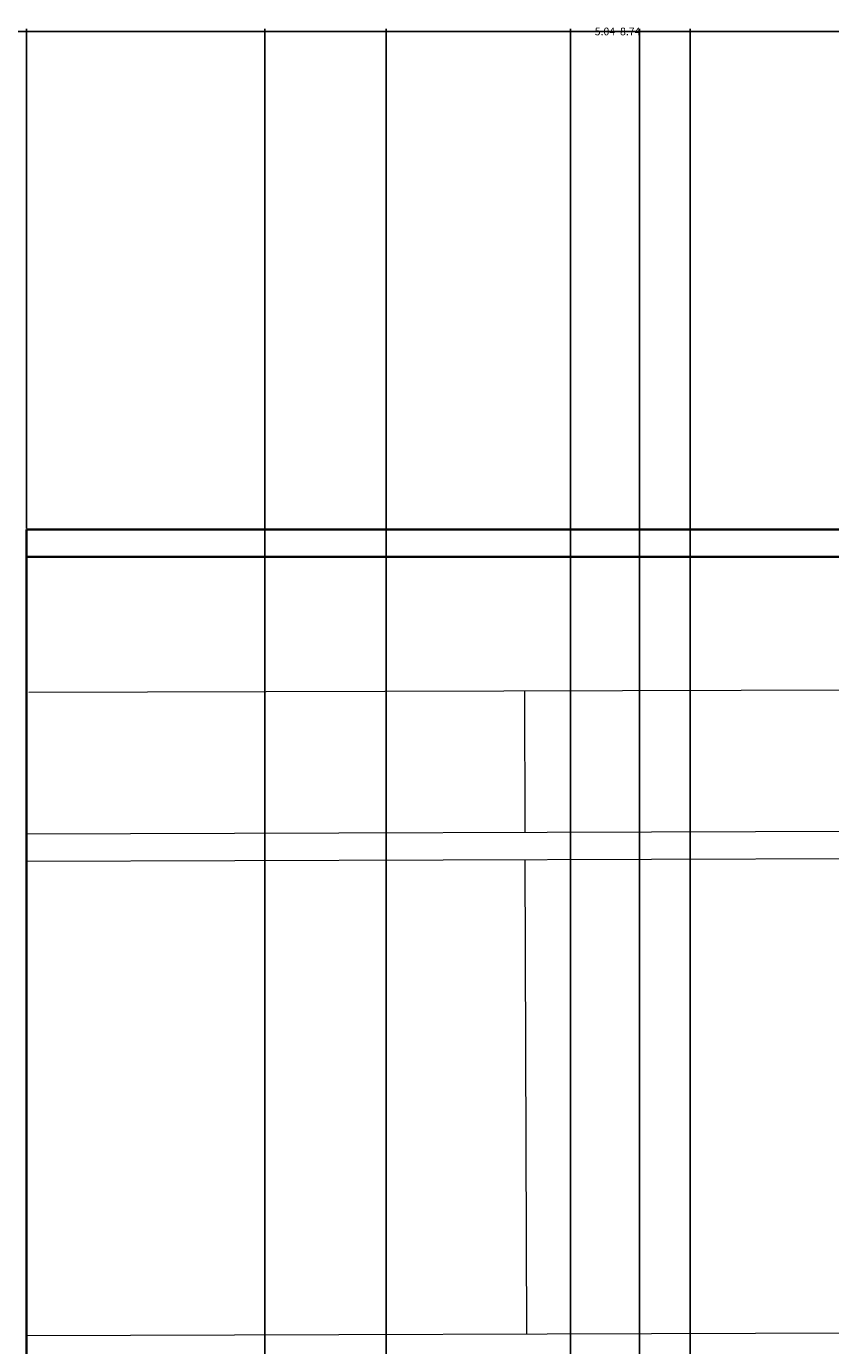
# Model space of a CAD drawing. Units: inches. Extents: x -26 to 776, y -22 to 650.
# Tile 36 of 62: x 192 to 250, y 554 to 650. Entities that reach past the tile are written whole.
import ezdxf

# ---------------------------------------------------------------- set-up
doc = ezdxf.new("R2010")
doc.units = ezdxf.units.IN
doc.header["$MEASUREMENT"] = 0
for name, color, linetype, lineweight in [('A-ANNO-DIMS', 2, 'Continuous', 18), ('A-ROOF', 7, 'Continuous', 35), ('A-WALL', 7, 'Continuous', 35), ('A-WALL-TRIM', 7, 'Continuous', 18)]:
    doc.layers.add(name, color=color, linetype=linetype, lineweight=lineweight)
doc.styles.get("Standard").update_dxf_attribs({"font": 'arial.ttf'})
doc.dimstyles.get("Standard").update_dxf_attribs({"dimtxt": 0.5625, "dimasz": 0.18, "dimexe": 0.18, "dimexo": 0.0625, "dimgap": 0.09, "dimtad": 0, "dimtih": 1, "dimtoh": 1, "dimdec": 4, "dimzin": 0, "dimdsep": 46, "dimlunit": 4, "dimtxsty": 'Standard', "dimcen": 0.09, "dimadec": 0, "dimazin": 0, "dimtfac": 1, "dimtdec": 4, "dimtofl": 0, "dimtmove": 0, "dimatfit": 3, "dimfxl": 1, "dimtolj": 1, "dimtzin": 0, "dimarcsym": 0})

# ---------------------------------------------------------------- blocks, each defined once
blk = doc.blocks.new('*D15')
at = {"layer": 'A-ANNO-DIMS', "color": 0, "lineweight": -2, "transparency": 16777216}
for p, q in [((11.107, 491.489), (11.107, 649.856)), ((11.287, 649.676), (120.222, 649.676)), ((231.245, 649.676), (122.31, 649.676)), ((231.425, 491.489), (231.425, 649.856))]:
    blk.add_line(p, q, dxfattribs=at)
at = {"layer": 'A-ANNO-DIMS', "color": 0, "transparency": 16777216}
for points in [[(11.287, 649.706), (11.287, 649.646), (11.107, 649.676)], [(231.245, 649.706), (231.245, 649.646), (231.425, 649.676)]]:
    blk.add_solid(points, dxfattribs=at)
at = {"layer": 'Defpoints', "color": 0, "transparency": 16777216}
for p in [(231.425, 649.676), (11.107, 491.427), (231.425, 491.427)]:
    blk.add_point(p, dxfattribs=at)
at = {"layer": 'A-ANNO-DIMS', "color": 0, "transparency": 16777216, "insert": (121.266, 649.676), "char_height": 0.5625, "attachment_point": 5}
blk.add_mtext('\\A1;220.3', dxfattribs=at)
blk = doc.blocks.new('*D16')
at = {"layer": 'A-ANNO-DIMS', "color": 0, "lineweight": -2, "transparency": 16777216}
for p, q in [((231.425, 504.483), (231.425, 649.856)), ((231.605, 649.676), (259.297, 649.676)), ((289.062, 649.676), (261.37, 649.676)), ((289.242, 504.483), (289.242, 649.856))]:
    blk.add_line(p, q, dxfattribs=at)
at = {"layer": 'A-ANNO-DIMS', "color": 0, "transparency": 16777216}
for points in [[(231.605, 649.706), (231.605, 649.646), (231.425, 649.676)], [(289.062, 649.706), (289.062, 649.646), (289.242, 649.676)]]:
    blk.add_solid(points, dxfattribs=at)
at = {"layer": 'Defpoints', "color": 0, "transparency": 16777216}
for p in [(289.242, 649.676), (231.425, 504.42), (289.242, 504.42)]:
    blk.add_point(p, dxfattribs=at)
at = {"layer": 'A-ANNO-DIMS', "color": 0, "transparency": 16777216, "insert": (260.334, 649.676), "char_height": 0.5625, "attachment_point": 5}
blk.add_mtext('\\A1;57.82', dxfattribs=at)
blk = doc.blocks.new('*D18')
at = {"layer": 'A-ANNO-DIMS', "color": 0, "lineweight": -2, "transparency": 16777216}
for p, q in [((191.678, 613.334), (191.678, 649.856)), ((191.858, 649.676), (273.361, 649.676)), ((356.887, 649.676), (275.384, 649.676)), ((357.067, 613.334), (357.067, 649.856))]:
    blk.add_line(p, q, dxfattribs=at)
at = {"layer": 'A-ANNO-DIMS', "color": 0, "transparency": 16777216}
for points in [[(191.858, 649.706), (191.858, 649.646), (191.678, 649.676)], [(356.887, 649.706), (356.887, 649.646), (357.067, 649.676)]]:
    blk.add_solid(points, dxfattribs=at)
at = {"layer": 'Defpoints', "color": 0, "transparency": 16777216}
for p in [(357.067, 649.676), (191.678, 613.271), (357.067, 613.271)]:
    blk.add_point(p, dxfattribs=at)
at = {"layer": 'A-ANNO-DIMS', "color": 0, "transparency": 16777216, "insert": (274.373, 649.676), "char_height": 0.5625, "attachment_point": 5}
blk.add_mtext('\\A1;165.4', dxfattribs=at)
blk = doc.blocks.new('*D22')
at = {"layer": 'A-ANNO-DIMS', "color": 0, "lineweight": -2, "transparency": 16777216}
for p, q in [((22.889, 15.333), (22.889, 649.856)), ((23.069, 649.676), (119.19, 649.676)), ((217.773, 649.676), (121.652, 649.676)), ((217.953, 15.545), (217.953, 649.856))]:
    blk.add_line(p, q, dxfattribs=at)
at = {"layer": 'A-ANNO-DIMS', "color": 0, "transparency": 16777216}
for points in [[(23.069, 649.706), (23.069, 649.646), (22.889, 649.676)], [(217.773, 649.706), (217.773, 649.646), (217.953, 649.676)]]:
    blk.add_solid(points, dxfattribs=at)
at = {"layer": 'Defpoints', "color": 0, "transparency": 16777216}
for p in [(217.953, 649.676), (217.953, 15.482), (22.889, 15.27)]:
    blk.add_point(p, dxfattribs=at)
at = {"layer": 'A-ANNO-DIMS', "color": 0, "transparency": 16777216, "insert": (120.421, 649.676), "char_height": 0.5625, "attachment_point": 5}
blk.add_mtext('\\A1;195.06', dxfattribs=at)
blk = doc.blocks.new('*D35')
at = {"layer": 'A-ANNO-DIMS', "color": 0, "lineweight": -2, "transparency": 16777216}
for p, q in [((82.134, 420.341), (82.134, 649.856)), ((82.314, 649.676), (144.382, 649.676)), ((208.911, 649.676), (146.843, 649.676)), ((209.091, 420.341), (209.091, 649.856))]:
    blk.add_line(p, q, dxfattribs=at)
at = {"layer": 'A-ANNO-DIMS', "color": 0, "transparency": 16777216}
for points in [[(82.314, 649.706), (82.314, 649.646), (82.134, 649.676)], [(208.911, 649.706), (208.911, 649.646), (209.091, 649.676)]]:
    blk.add_solid(points, dxfattribs=at)
at = {"layer": 'Defpoints', "color": 0, "transparency": 16777216}
for p in [(209.091, 649.676), (82.134, 420.278), (209.091, 420.278)]:
    blk.add_point(p, dxfattribs=at)
at = {"layer": 'A-ANNO-DIMS', "color": 0, "transparency": 16777216, "insert": (145.613, 649.676), "char_height": 0.5625, "attachment_point": 5}
blk.add_mtext('\\A1;126.96', dxfattribs=at)
blk = doc.blocks.new('*D43')
at = {"layer": 'A-ANNO-DIMS', "color": 0, "lineweight": -2, "transparency": 16777216}
for p, q in [((231.425, 159.545), (231.425, 649.856)), ((231.605, 649.676), (233.125, 649.676)), ((236.285, 649.676), (234.764, 649.676)), ((236.465, 171.48), (236.465, 649.856))]:
    blk.add_line(p, q, dxfattribs=at)
at = {"layer": 'A-ANNO-DIMS', "color": 0, "transparency": 16777216}
for points in [[(231.605, 649.706), (231.605, 649.646), (231.425, 649.676)], [(236.285, 649.706), (236.285, 649.646), (236.465, 649.676)]]:
    blk.add_solid(points, dxfattribs=at)
at = {"layer": 'Defpoints', "color": 0, "transparency": 16777216}
for p in [(236.465, 649.676), (236.465, 171.417), (231.425, 159.482)]:
    blk.add_point(p, dxfattribs=at)
at = {"layer": 'A-ANNO-DIMS', "color": 0, "transparency": 16777216, "insert": (233.945, 649.676), "char_height": 0.5625, "attachment_point": 5}
blk.add_mtext('\\A1;5.04', dxfattribs=at)
blk = doc.blocks.new('*D44')
at = {"layer": 'A-ANNO-DIMS', "color": 0, "lineweight": -2, "transparency": 16777216}
for p, q in [((231.425, 15.545), (231.425, 649.856)), ((231.605, 649.676), (234.975, 649.676)), ((239.985, 649.676), (236.615, 649.676)), ((240.165, 26.486), (240.165, 649.856))]:
    blk.add_line(p, q, dxfattribs=at)
at = {"layer": 'A-ANNO-DIMS', "color": 0, "transparency": 16777216}
for points in [[(231.605, 649.706), (231.605, 649.646), (231.425, 649.676)], [(239.985, 649.706), (239.985, 649.646), (240.165, 649.676)]]:
    blk.add_solid(points, dxfattribs=at)
at = {"layer": 'Defpoints', "color": 0, "transparency": 16777216}
for p in [(240.165, 649.676), (240.165, 26.424), (231.425, 15.482)]:
    blk.add_point(p, dxfattribs=at)
at = {"layer": 'A-ANNO-DIMS', "color": 0, "transparency": 16777216, "insert": (235.795, 649.676), "char_height": 0.5625, "attachment_point": 5}
blk.add_mtext('\\A1;8.74', dxfattribs=at)

msp = doc.modelspace()

# ---------------------------------------------------------------- linework, layer by layer
at = {"layer": 'A-ROOF'}
for p, q in [((191.6782, 613.2713), (357.0669, 613.2713)), ((191.6782, 611.2713), (357.0669, 611.2713))]:
    msp.add_line(p, q, dxfattribs=at)
at = {"layer": 'A-WALL'}
msp.add_line((191.6782, 491.4269), (191.6782, 613.2713), dxfattribs=at)
at = {"layer": 'A-WALL-TRIM'}
for p, q in [((191.8658, 601.3674), (357.1028, 601.8885)), ((228.062, 601.4816), (228.0946, 591.1471)), ((191.6719, 591.0323), (357.2511, 591.5545)), ((191.6782, 589.0323), (357.2574, 589.5545)), ((228.1009, 589.1472), (228.2103, 554.4643)), ((191.6719, 554.3491), (357.2511, 554.8713))]:
    msp.add_line(p, q, dxfattribs=at)

# ---------------------------------------------------------------- dimensions: what is measured, and where the dimension line sits
at = {"layer": 'A-ANNO-DIMS'}
for base, p1, p2, override, picture, middle in [((231.4249, 649.6763), (11.1074, 491.4269), (231.4249, 491.4269), {"dimdec": 1, "dimlfac": 1, "dimrnd": 0, "dimzin": 0, "dimdsep": 46, "dimlunit": 2}, '*D15', (121.2661, 649.6763)), ((217.9529, 649.6763), (22.8891, 15.2701), (217.9529, 15.4824), {"dimdec": 2, "dimlfac": 1, "dimrnd": 0, "dimzin": 0, "dimdsep": 46, "dimlunit": 2}, '*D22', (120.421, 649.6763)), ((209.091, 649.6763), (82.134, 420.2783), (209.091, 420.2783), {"dimdec": 2, "dimlfac": 1, "dimrnd": 0, "dimzin": 0, "dimdsep": 46, "dimlunit": 2}, '*D35', (145.6125, 649.6763)), ((357.0669, 649.6763), (191.6782, 613.2713), (357.0669, 613.2713), {"dimdec": 1, "dimlfac": 1, "dimrnd": 0, "dimzin": 0, "dimdsep": 46, "dimlunit": 2}, '*D18', (274.3725, 649.6763)), ((289.2424, 649.6763), (231.4249, 504.4205), (289.2424, 504.4205), {"dimdec": 2, "dimlfac": 1, "dimrnd": 0, "dimzin": 0, "dimdsep": 46, "dimlunit": 2}, '*D16', (260.3336, 649.6763)), ((236.4647, 649.6763), (231.4249, 159.4824), (236.4647, 171.4173), {"dimdec": 2, "dimlfac": 1, "dimrnd": 0, "dimzin": 0, "dimdsep": 46, "dimlunit": 2}, '*D43', (233.9448, 649.6763)), ((240.1654, 649.6763), (231.4249, 15.4824), (240.1654, 26.4239), {"dimdec": 2, "dimlfac": 1, "dimrnd": 0, "dimzin": 0, "dimdsep": 46, "dimlunit": 2}, '*D44', (235.7952, 649.6763))]:
    dim = msp.add_linear_dim(base=base, p1=p1, p2=p2, dimstyle='Standard', override=override, dxfattribs=at)
    dim.commit()
    dim.dimension.update_dxf_attribs({"geometry": picture, "text_midpoint": middle})

doc.saveas('drawing.dxf')
